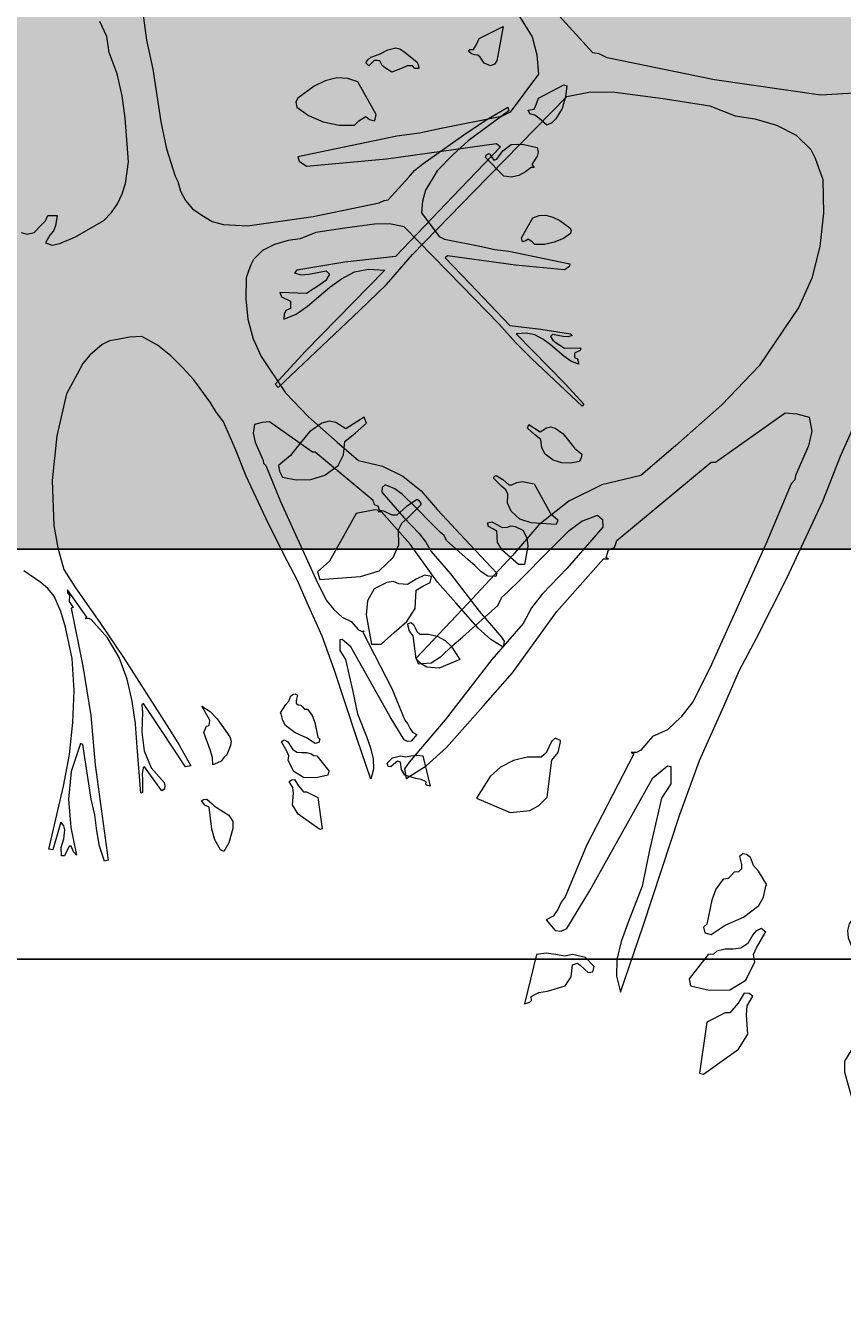
# Model space of a CAD drawing. Units: inches. Extents: x 84 to 1044, y -280 to 906.
# Tile 24 of 105: x 721 to 739, y -129 to -101. Entities that reach past the tile are written whole.
import ezdxf

# ---------------------------------------------------------------- set-up
doc = ezdxf.new("R2010")
doc.units = ezdxf.units.IN
for name, color, linetype, lineweight in [('A-ANNO-DIMS', 2, 'Continuous', 18), ('C-PROP', 7, 'Continuous', 25), ('L-PLNT', 114, 'Continuous', 15)]:
    doc.layers.add(name, color=color, linetype=linetype, lineweight=lineweight)
doc.layers.add('L-PLNT-PATT', color=9, linetype='Continuous', lineweight=9, true_color=0xafd9aa)
doc.styles.get("Standard").update_dxf_attribs({"font": 'arial.ttf'})
doc.dimstyles.get("Standard").update_dxf_attribs({"dimtxt": 0.18, "dimasz": 0.18, "dimexe": 0.18, "dimexo": 0.0625, "dimgap": 0.09, "dimtad": 0, "dimtih": 1, "dimtoh": 1, "dimdec": 4, "dimzin": 0, "dimdsep": 46, "dimtxsty": 'Standard', "dimcen": 0.09, "dimadec": 0, "dimazin": 0, "dimtfac": 1, "dimtdec": 4, "dimtofl": 0, "dimtmove": 0, "dimatfit": 3, "dimfxl": 1, "dimtolj": 1, "dimtzin": 0, "dimarcsym": 0})

# ---------------------------------------------------------------- blocks, each defined once
blk = doc.blocks.new('A$C37E508DF')
for p, q in [((0.7761, 1.2285), (0.7821, 1.1856)), ((0.7246, 1.1908), (0.7148, 1.2126)), ((1.2628, 1.1882), (1.2975, 1.2053)), ((1.2975, 1.2053), (1.2885, 1.1556)), ((0.7281, 1.168), (0.7246, 1.1908)), ((0.7821, 1.1856), (0.7911, 1.1436)), ((1.2589, 1.1792), (1.2628, 1.1882)), ((0.7396, 1.1371), (0.7281, 1.168)), ((1.1187, 1.1655), (1.1307, 1.1714)), ((1.1307, 1.1714), (1.1423, 1.1744)), ((1.1423, 1.1744), (1.1483, 1.1732)), ((1.1483, 1.1732), (1.1539, 1.1693)), ((1.1539, 1.1693), (1.1727, 1.1543)), ((1.2469, 1.1702), (1.2495, 1.1723)), ((1.2478, 1.1693), (1.2469, 1.1702)), ((1.2516, 1.1659), (1.2478, 1.1693)), ((1.2495, 1.1723), (1.2546, 1.1719)), ((1.2546, 1.1719), (1.2589, 1.1792)), ((1.099, 1.153), (1.102, 1.1573)), ((1.102, 1.1573), (1.1063, 1.1612)), ((1.1063, 1.1612), (1.1187, 1.1655)), ((1.2563, 1.1646), (1.2516, 1.1659)), ((1.2611, 1.1637), (1.2563, 1.1646)), ((1.2641, 1.1612), (1.2611, 1.1637)), ((1.2701, 1.1522), (1.2641, 1.1612)), ((1.1033, 1.1487), (1.099, 1.153)), ((1.111, 1.156), (1.1033, 1.1487)), ((1.1153, 1.1564), (1.111, 1.156)), ((1.1191, 1.1556), (1.1153, 1.1564)), ((1.1226, 1.1492), (1.1191, 1.1556)), ((1.1273, 1.1453), (1.1226, 1.1492)), ((1.1367, 1.1393), (1.1273, 1.1453)), ((1.1517, 1.1453), (1.1367, 1.1393)), ((1.1586, 1.1483), (1.1517, 1.1453)), ((1.1663, 1.1487), (1.1586, 1.1483)), ((1.1697, 1.1449), (1.1663, 1.1487)), ((1.1727, 1.1543), (1.1749, 1.1504)), ((1.1749, 1.1504), (1.1757, 1.1449)), ((1.2791, 1.1487), (1.2701, 1.1522)), ((1.2851, 1.1509), (1.2791, 1.1487)), ((1.2885, 1.1556), (1.2851, 1.1509)), ((0.7469, 1.1054), (0.7396, 1.1371)), ((0.7911, 1.1436), (0.8027, 1.0677)), ((1.1757, 1.1449), (1.1697, 1.1449)), ((1.3485, 1.102), (1.385, 1.1209)), ((1.385, 1.1209), (1.3897, 1.1196)), ((1.3897, 1.1196), (1.3875, 1.1037)), ((0.7512, 1.0728), (0.7469, 1.1054)), ((1.3455, 1.0934), (1.3485, 1.102)), ((1.3875, 1.1037), (1.3828, 1.087)), ((1.2713, 1.0694), (1.3044, 1.0887)), ((1.3044, 1.0887), (1.3057, 1.0835)), ((1.3421, 1.0861), (1.3455, 1.0934)), ((1.3057, 1.0835), (1.2469, 1.0402)), ((1.3335, 1.0844), (1.3421, 1.0861)), ((1.3361, 1.0793), (1.3335, 1.0844)), ((1.3434, 1.0771), (1.3361, 1.0793)), ((1.3828, 1.087), (1.3738, 1.072)), ((0.7538, 1.0415), (0.7512, 1.0728)), ((0.8027, 1.0677), (0.8108, 1.0287)), ((1.2409, 1.0488), (1.2713, 1.0694)), ((1.349, 1.0728), (1.3434, 1.0771)), ((1.3605, 1.063), (1.349, 1.0728)), ((1.3678, 1.0664), (1.3605, 1.063)), ((1.3738, 1.072), (1.3678, 1.0664)), ((1.1813, 1.0072), (1.2409, 1.0488)), ((0.7559, 1.0098), (0.7538, 1.0415)), ((1.2469, 1.0402), (1.2246, 1.0201)), ((1.2971, 1.0257), (1.3091, 1.0351)), ((1.3091, 1.0351), (1.3185, 1.0355)), ((1.3185, 1.0355), (1.3275, 1.0347)), ((1.3275, 1.0347), (1.3468, 1.0308)), ((0.8108, 1.0287), (0.8233, 0.9892)), ((1.2731, 1.0197), (1.2761, 1.0218)), ((1.2761, 1.0218), (1.2786, 1.0209)), ((1.2786, 1.0209), (1.2799, 1.0184)), ((1.2885, 1.0136), (1.2971, 1.0257)), ((1.3468, 1.0308), (1.3481, 1.0239)), ((1.3481, 1.0239), (1.3468, 1.018)), ((0.7516, 0.9785), (0.7559, 1.0098)), ((1.2246, 1.0201), (1.2023, 0.9969)), ((1.2718, 1.0162), (1.2731, 1.0197)), ((1.2984, 0.9892), (1.2718, 1.0162)), ((1.2799, 1.0184), (1.2842, 1.0124)), ((1.2842, 1.0124), (1.2885, 1.0136)), ((1.3468, 1.018), (1.3391, 1.0059)), ((1.1693, 0.9974), (1.1813, 1.0072)), ((1.3378, 1.0016), (1.3297, 0.9952)), ((1.3421, 1.0016), (1.3378, 1.0016)), ((1.3391, 1.0059), (1.3421, 1.0016)), ((0.8233, 0.9892), (0.8275, 0.9815)), ((1.1311, 0.9549), (1.1612, 0.9879)), ((1.1612, 0.9879), (1.1693, 0.9974)), ((1.2023, 0.9969), (1.1852, 0.9691)), ((1.3095, 0.9875), (1.2984, 0.9892)), ((1.3202, 0.9901), (1.3095, 0.9875)), ((1.3297, 0.9952), (1.3202, 0.9901)), ((0.7469, 0.9635), (0.7516, 0.9785)), ((0.8275, 0.9815), (0.8314, 0.9673)), ((0.8314, 0.9673), (0.8383, 0.954)), ((1.1852, 0.9691), (1.1809, 0.9532)), ((0.7401, 0.9493), (0.7469, 0.9635)), ((0.8383, 0.954), (0.8486, 0.942)), ((1.1183, 0.9506), (1.1256, 0.954)), ((1.1256, 0.954), (1.1311, 0.9549)), ((1.1809, 0.9532), (1.1796, 0.936)), ((0.7315, 0.9365), (0.7401, 0.9493)), ((0.8486, 0.942), (0.8619, 0.933)), ((1.0227, 0.9309), (1.1183, 0.9506)), ((0.6359, 0.9245), (0.6397, 0.9322)), ((0.6397, 0.9322), (0.653, 0.9322)), ((0.653, 0.9322), (0.6505, 0.9172)), ((0.7203, 0.9253), (0.7315, 0.9365)), ((0.8619, 0.933), (0.8769, 0.9236)), ((0.9279, 0.9172), (1.0227, 0.9309)), ((1.1796, 0.936), (1.2049, 0.9022)), ((1.3404, 0.9292), (1.3494, 0.9322)), ((1.3494, 0.9322), (1.3592, 0.9326)), ((1.3592, 0.9326), (1.3695, 0.93)), ((1.3695, 0.93), (1.3794, 0.9253)), ((0.6196, 0.9077), (0.6303, 0.9189)), ((0.6303, 0.9189), (0.6359, 0.9245)), ((0.6796, 0.9013), (0.7203, 0.9253)), ((0.8769, 0.9236), (0.8936, 0.9193)), ((0.8936, 0.9193), (0.9279, 0.9172)), ((1.1114, 0.9198), (1.0685, 0.9142)), ((1.1333, 0.9202), (1.1114, 0.9198)), ((1.1543, 0.9159), (1.1333, 0.9202)), ((1.3241, 0.9), (1.3404, 0.9292)), ((1.3794, 0.9253), (1.394, 0.9146)), ((0.6011, 0.9077), (0.6097, 0.9056)), ((0.6097, 0.9056), (0.6196, 0.9077)), ((0.6479, 0.9103), (0.6423, 0.9039)), ((0.6505, 0.9172), (0.6479, 0.9103)), ((1.0269, 0.9077), (1.0042, 0.8987)), ((1.0685, 0.9142), (1.0269, 0.9077)), ((1.2371, 0.8314), (1.1543, 0.9159)), ((1.394, 0.9146), (1.3957, 0.9112)), ((1.3957, 0.9112), (1.3948, 0.9065)), ((0.6384, 0.8974), (0.6359, 0.8927)), ((0.6423, 0.9039), (0.6384, 0.8974)), ((0.6569, 0.8919), (0.6796, 0.9013)), ((0.9866, 0.8962), (0.9673, 0.8906)), ((1.0042, 0.8987), (0.9866, 0.8962)), ((1.2049, 0.9022), (1.2126, 0.8983)), ((1.2126, 0.8983), (1.2662, 0.8876)), ((1.3254, 0.8944), (1.3241, 0.9)), ((1.3301, 0.8957), (1.3254, 0.8944)), ((1.3335, 0.8983), (1.3301, 0.8957)), ((1.3395, 0.8944), (1.3335, 0.8983)), ((1.3846, 0.8992), (1.3713, 0.8936)), ((1.3948, 0.9065), (1.3846, 0.8992)), ((0.6359, 0.8927), (0.6457, 0.8897)), ((0.6457, 0.8897), (0.6569, 0.8919)), ((0.9673, 0.8906), (0.9498, 0.8816)), ((1.2662, 0.8876), (1.2855, 0.8833)), ((1.3434, 0.8906), (1.3395, 0.8944)), ((1.3571, 0.8906), (1.3434, 0.8906)), ((1.3713, 0.8936), (1.3571, 0.8906)), ((0.9498, 0.8816), (0.9369, 0.8687)), ((1.2169, 0.8743), (1.2135, 0.8713)), ((1.3151, 0.8606), (1.2169, 0.8743)), ((1.2855, 0.8833), (1.3057, 0.8807)), ((1.3057, 0.8807), (1.394, 0.8623)), ((0.9369, 0.8687), (0.933, 0.861)), ((1.2135, 0.8713), (1.2491, 0.834)), ((1.394, 0.8623), (1.3927, 0.8584)), ((0.9296, 0.852), (0.9262, 0.8421)), ((0.933, 0.861), (0.9296, 0.852)), ((1.3863, 0.8541), (1.3151, 0.8606)), ((1.3927, 0.8584), (1.3863, 0.8541)), ((0.9262, 0.8421), (0.9257, 0.8121)), ((1.2919, 0.7752), (1.2371, 0.8314)), ((1.2491, 0.834), (1.3069, 0.7735)), ((0.9257, 0.8121), (0.9287, 0.7825)), ((0.9287, 0.7825), (0.936, 0.7542)), ((1.3151, 0.7487), (1.2919, 0.7752)), ((1.3069, 0.7735), (1.352, 0.7684)), ((1.3309, 0.7624), (1.3164, 0.7615)), ((1.3164, 0.7615), (1.3871, 0.6891)), ((1.3434, 0.7598), (1.3309, 0.7624)), ((1.355, 0.7538), (1.3434, 0.7598)), ((1.352, 0.7684), (1.3948, 0.7615)), ((1.3687, 0.7607), (1.3657, 0.7577)), ((1.3841, 0.7577), (1.3687, 0.7607)), ((1.3948, 0.7615), (1.397, 0.759)), ((0.7285, 0.7512), (0.7182, 0.7461)), ((0.7401, 0.7534), (0.7285, 0.7512)), ((0.7577, 0.7568), (0.7401, 0.7534)), ((0.7752, 0.7577), (0.7577, 0.7568)), ((0.798, 0.7452), (0.7752, 0.7577)), ((0.936, 0.7542), (0.9476, 0.7285)), ((1.3391, 0.7255), (1.3151, 0.7487)), ((1.3653, 0.7461), (1.355, 0.7538)), ((1.3657, 0.7577), (1.3691, 0.7521)), ((1.3691, 0.7521), (1.3743, 0.7482)), ((1.3914, 0.7572), (1.3841, 0.7577)), ((1.397, 0.759), (1.3914, 0.7572)), ((0.7182, 0.7461), (0.7002, 0.7307)), ((0.8173, 0.7298), (0.798, 0.7452)), ((1.3854, 0.7294), (1.3653, 0.7461)), ((1.3743, 0.7482), (1.3863, 0.7405)), ((1.3863, 0.7405), (1.4099, 0.7414)), ((1.4086, 0.7375), (1.4004, 0.7337)), ((1.4099, 0.7414), (1.4086, 0.7375)), ((0.7002, 0.7307), (0.6903, 0.7186)), ((0.8344, 0.7122), (0.8173, 0.7298)), ((0.9476, 0.7285), (0.9828, 0.6762)), ((1.3953, 0.7221), (1.3854, 0.7294)), ((1.4004, 0.7337), (1.4004, 0.7272)), ((1.4004, 0.7272), (1.4047, 0.7255)), ((0.6903, 0.7186), (0.6818, 0.7032)), ((1.4116, 0.6569), (1.3391, 0.7255)), ((1.4064, 0.7178), (1.3953, 0.7221)), ((1.4047, 0.7255), (1.406, 0.7221)), ((1.406, 0.7221), (1.4064, 0.7178)), ((0.6818, 0.7032), (0.6667, 0.6749)), ((0.8503, 0.6951), (0.8344, 0.7122)), ((0.8739, 0.6629), (0.8503, 0.6951)), ((1.3871, 0.6891), (1.4141, 0.6599)), ((0.6667, 0.6749), (0.6526, 0.614)), ((0.9828, 0.6762), (1.0162, 0.6415)), ((0.8824, 0.6492), (0.8739, 0.6629)), ((1.4141, 0.6599), (1.4116, 0.6569)), ((0.8932, 0.6342), (0.8824, 0.6492)), ((1.0162, 0.6415), (1.0574, 0.605)), ((0.9103, 0.5956), (0.8932, 0.6342)), ((0.9382, 0.6303), (0.936, 0.6179)), ((0.9493, 0.6333), (0.9382, 0.6303)), ((0.9596, 0.6342), (0.9493, 0.6333)), ((1.0218, 0.5904), (0.9596, 0.6342)), ((1.3327, 0.6252), (1.3348, 0.6303)), ((1.343, 0.6162), (1.3327, 0.6252)), ((1.3348, 0.6303), (1.3511, 0.62)), ((1.3511, 0.62), (1.3601, 0.6256)), ((1.3601, 0.6256), (1.3661, 0.6269)), ((1.3661, 0.6269), (1.3725, 0.6252)), ((1.3725, 0.6252), (1.3837, 0.6175)), ((0.6526, 0.614), (0.6457, 0.5497)), ((0.936, 0.6179), (0.939, 0.605)), ((1.352, 0.6089), (1.343, 0.6162)), ((1.3837, 0.6175), (1.3918, 0.6072)), ((0.939, 0.605), (0.9506, 0.5784)), ((1.0574, 0.605), (1.0883, 0.5784)), ((1.3533, 0.5969), (1.352, 0.6089)), ((1.3918, 0.6072), (1.4004, 0.5964)), ((0.9262, 0.5557), (0.9103, 0.5956)), ((1.0256, 0.5904), (1.0218, 0.5904)), ((1.1097, 0.5205), (1.0256, 0.5904)), ((1.358, 0.5874), (1.3533, 0.5969)), ((1.4004, 0.5964), (1.4111, 0.5874)), ((0.9506, 0.5784), (0.951, 0.5746)), ((1.0883, 0.5784), (1.123, 0.5703)), ((1.37, 0.5789), (1.358, 0.5874)), ((1.3824, 0.575), (1.37, 0.5789)), ((1.4103, 0.5823), (1.4077, 0.5771)), ((1.4111, 0.5874), (1.4103, 0.5823)), ((0.951, 0.5746), (0.9545, 0.5711)), ((0.9545, 0.5711), (0.9759, 0.5193)), ((1.123, 0.5703), (1.1526, 0.5557)), ((1.3953, 0.5746), (1.3824, 0.575)), ((1.4077, 0.5771), (1.3953, 0.5746)), ((0.9583, 0.4871), (0.9262, 0.5557)), ((1.1526, 0.5557), (1.1792, 0.5347)), ((1.2842, 0.554), (1.2855, 0.5557)), ((1.2855, 0.5557), (1.2876, 0.557)), ((1.2876, 0.557), (1.2971, 0.551)), ((0.6457, 0.5497), (0.6483, 0.4845)), ((1.2842, 0.5527), (1.2842, 0.554)), ((1.2958, 0.5407), (1.2842, 0.5527)), ((1.2971, 0.551), (1.3057, 0.5433)), ((1.3099, 0.5433), (1.3172, 0.5467)), ((1.3172, 0.5467), (1.3254, 0.548)), ((1.3254, 0.548), (1.3421, 0.5446)), ((1.3421, 0.5446), (1.3657, 0.5021)), ((1.1226, 0.5394), (1.1221, 0.5325)), ((1.1268, 0.5433), (1.1226, 0.5394)), ((1.141, 0.5377), (1.1268, 0.5433)), ((1.1521, 0.5296), (1.141, 0.5377)), ((1.1792, 0.5347), (1.2027, 0.5072)), ((1.3014, 0.536), (1.2958, 0.5407)), ((1.3044, 0.53), (1.3014, 0.536)), ((1.3057, 0.5433), (1.3099, 0.5433)), ((1.1221, 0.5325), (1.1539, 0.4961)), ((1.1706, 0.5111), (1.1521, 0.5296)), ((1.3039, 0.5167), (1.3044, 0.53)), ((0.9759, 0.5193), (1.0269, 0.4069)), ((1.1118, 0.5145), (1.1097, 0.5205)), ((1.117, 0.5124), (1.1118, 0.5145)), ((1.1191, 0.5055), (1.117, 0.5124)), ((1.1955, 0.4858), (1.1706, 0.5111)), ((1.3091, 0.5055), (1.3039, 0.5167)), ((1.117, 0.5042), (1.1191, 0.5055)), ((1.1217, 0.5042), (1.117, 0.5042)), ((1.1633, 0.4575), (1.1217, 0.5042)), ((1.2027, 0.5072), (1.2426, 0.4644)), ((1.3215, 0.4935), (1.3091, 0.5055)), ((1.3657, 0.5021), (1.3764, 0.4927)), ((1.1539, 0.4961), (1.1762, 0.4729)), ((1.2748, 0.4884), (1.2812, 0.4897)), ((1.2761, 0.4832), (1.2748, 0.4884)), ((1.2812, 0.4897), (1.2885, 0.4862)), ((1.3382, 0.4884), (1.3215, 0.4935)), ((1.3743, 0.4858), (1.3382, 0.4884)), ((1.3764, 0.4927), (1.3743, 0.4858)), ((0.6483, 0.4845), (0.6539, 0.4524)), ((0.9853, 0.4335), (0.9583, 0.4871)), ((1.207, 0.4747), (1.1955, 0.4858)), ((1.2825, 0.4798), (1.2761, 0.4832)), ((1.2885, 0.4764), (1.2825, 0.4798)), ((1.2885, 0.4862), (1.2962, 0.4815)), ((1.2894, 0.4601), (1.2885, 0.4764)), ((1.2962, 0.4815), (1.3039, 0.482)), ((1.3039, 0.482), (1.3087, 0.4841)), ((1.3087, 0.4841), (1.3147, 0.4832)), ((1.3147, 0.4832), (1.3258, 0.4777)), ((1.3258, 0.4777), (1.3318, 0.4669)), ((1.1762, 0.4729), (1.1856, 0.4605)), ((1.2122, 0.47), (1.207, 0.4747)), ((1.2156, 0.4627), (1.2122, 0.47)), ((1.3318, 0.4669), (1.3331, 0.4545)), ((1.2027, 0.4026), (1.1633, 0.4575)), ((1.1856, 0.4605), (1.1933, 0.4468)), ((1.2469, 0.4348), (1.2156, 0.4627)), ((1.2426, 0.4644), (1.2885, 0.4159)), ((1.2967, 0.4485), (1.2894, 0.4601)), ((1.3331, 0.4545), (1.3284, 0.4284)), ((0.6539, 0.4524), (0.6625, 0.4211)), ((1.1933, 0.4468), (1.2212, 0.4146)), ((1.3082, 0.4386), (1.2967, 0.4485)), ((1.0003, 0.4052), (0.9853, 0.4335)), ((1.2568, 0.4266), (1.2469, 0.4348)), ((1.3198, 0.4284), (1.3082, 0.4386)), ((0.6625, 0.4211), (0.6796, 0.3945)), ((1.2658, 0.4176), (1.2568, 0.4266)), ((1.3284, 0.4284), (1.3198, 0.4284)), ((0.6295, 0.4022), (0.6046, 0.4189)), ((1.2212, 0.4146), (1.2628, 0.361)), ((1.2752, 0.4116), (1.2658, 0.4176)), ((1.2868, 0.4108), (1.2752, 0.4116)), ((1.2885, 0.4159), (1.2868, 0.4108)), ((0.6397, 0.3936), (0.6295, 0.4022)), ((1.0145, 0.373), (1.0003, 0.4052)), ((1.0269, 0.4069), (1.0419, 0.3769)), ((1.2289, 0.373), (1.2027, 0.4026)), ((0.6487, 0.3825), (0.6397, 0.3936)), ((0.6959, 0.352), (0.668, 0.3919)), ((0.668, 0.3919), (0.668, 0.3872)), ((0.668, 0.3872), (0.6706, 0.3842)), ((0.6796, 0.3945), (0.7148, 0.3447)), ((0.6582, 0.3602), (0.6487, 0.3825)), ((0.6706, 0.3842), (0.6702, 0.3748)), ((0.6702, 0.3748), (0.6762, 0.3662)), ((1.0419, 0.3769), (1.0527, 0.3632)), ((0.6762, 0.3662), (0.6732, 0.3653)), ((0.6732, 0.3653), (0.6903, 0.2813)), ((1.0359, 0.3246), (1.0145, 0.373)), ((1.0527, 0.3632), (1.0647, 0.352)), ((1.2615, 0.3362), (1.2289, 0.373)), ((0.665, 0.3379), (0.6582, 0.3602)), ((0.6933, 0.3503), (0.6959, 0.352)), ((1.0647, 0.352), (1.078, 0.346)), ((1.2628, 0.361), (1.2949, 0.3233)), ((0.6985, 0.3503), (0.6933, 0.3503)), ((0.7023, 0.349), (0.6985, 0.3503)), ((0.7259, 0.3224), (0.7023, 0.349)), ((0.7148, 0.3447), (0.7487, 0.2937)), ((1.078, 0.346), (1.0883, 0.334)), ((1.1599, 0.3426), (1.1646, 0.3447)), ((1.1599, 0.3413), (1.1599, 0.3426)), ((1.162, 0.3319), (1.1599, 0.3413)), ((1.1646, 0.3447), (1.168, 0.3417)), ((1.168, 0.3417), (1.1702, 0.3366)), ((0.6745, 0.2924), (0.665, 0.3379)), ((1.0883, 0.334), (1.0921, 0.3319)), ((1.0921, 0.3319), (1.0968, 0.3319)), ((1.0968, 0.3319), (1.0947, 0.3306)), ((1.0947, 0.3306), (1.1367, 0.2491)), ((1.1676, 0.325), (1.162, 0.3319)), ((1.1702, 0.3366), (1.1727, 0.3314)), ((1.1727, 0.3314), (1.177, 0.3276)), ((1.2795, 0.3199), (1.2615, 0.3362)), ((0.7427, 0.2937), (0.7259, 0.3224)), ((1.0535, 0.2766), (1.0359, 0.3246)), ((1.0647, 0.3199), (1.0617, 0.3194)), ((1.0617, 0.3194), (1.0617, 0.304)), ((1.0711, 0.3147), (1.0647, 0.3199)), ((1.1719, 0.292), (1.1676, 0.325)), ((1.177, 0.3276), (1.1895, 0.3276)), ((1.1895, 0.3276), (1.2019, 0.3246)), ((1.2019, 0.3246), (1.2135, 0.3186)), ((1.2135, 0.3186), (1.2225, 0.3104)), ((1.2975, 0.3087), (1.2795, 0.3199)), ((1.2949, 0.3233), (1.2988, 0.3173)), ((1.0775, 0.3092), (1.0711, 0.3147)), ((1.1341, 0.2084), (1.0775, 0.3092)), ((1.2225, 0.3104), (1.2349, 0.2911)), ((1.2988, 0.3173), (1.2975, 0.3087)), ((1.0617, 0.304), (1.0698, 0.2911)), ((0.6775, 0.2465), (0.6745, 0.2924)), ((0.7542, 0.2628), (0.7427, 0.2937)), ((0.7487, 0.2937), (0.8151, 0.1899)), ((1.0698, 0.2911), (1.0805, 0.2448)), ((1.1792, 0.2847), (1.1719, 0.292)), ((1.1873, 0.28), (1.1792, 0.2847)), ((1.2349, 0.2911), (1.2049, 0.2783)), ((0.6903, 0.2813), (0.7015, 0.2101)), ((1.0861, 0.1775), (1.0535, 0.2766)), ((1.2049, 0.2783), (1.1873, 0.28)), ((0.7615, 0.2311), (0.7542, 0.2628)), ((0.6758, 0.2002), (0.6775, 0.2465)), ((0.9879, 0.2311), (0.9905, 0.2384)), ((0.9905, 0.2384), (0.9943, 0.241)), ((0.9943, 0.241), (0.9973, 0.2414)), ((0.9973, 0.2414), (1.0003, 0.2393)), ((1.0003, 0.2393), (0.9986, 0.232)), ((1.0805, 0.2448), (1.087, 0.2127)), ((1.1367, 0.2491), (1.1556, 0.2032)), ((0.7662, 0.1981), (0.7615, 0.2311)), ((0.7778, 0.2277), (0.7752, 0.2255)), ((0.8018, 0.1912), (0.7778, 0.2277)), ((0.9836, 0.226), (0.9879, 0.2311)), ((0.9986, 0.232), (0.9986, 0.2281)), ((0.9986, 0.2281), (1.0012, 0.2255)), ((0.7752, 0.2255), (0.7761, 0.2152)), ((0.8619, 0.2234), (0.8739, 0.2161)), ((0.87, 0.2101), (0.8619, 0.2234)), ((0.8739, 0.2161), (0.8841, 0.2054)), ((0.9759, 0.214), (0.9836, 0.226)), ((1.0012, 0.2255), (1.0051, 0.2251)), ((1.0051, 0.2251), (1.0076, 0.2225)), ((1.0076, 0.2225), (1.0106, 0.2195)), ((1.0106, 0.2195), (1.0149, 0.2191)), ((1.0149, 0.2191), (1.0214, 0.2101)), ((0.7015, 0.2101), (0.7079, 0.1389)), ((0.7761, 0.2152), (0.7752, 0.1861)), ((0.8734, 0.2032), (0.87, 0.2101)), ((0.8841, 0.2054), (0.9026, 0.1792)), ((0.9768, 0.2127), (0.9759, 0.214)), ((0.9789, 0.2028), (0.9768, 0.2127)), ((1.0214, 0.2101), (1.0252, 0.2002)), ((1.087, 0.2127), (1.0998, 0.1797)), ((1.1543, 0.1749), (1.1341, 0.2084)), ((0.6706, 0.1539), (0.6758, 0.2002)), ((0.7688, 0.1646), (0.7662, 0.1981)), ((0.8649, 0.1857), (0.8687, 0.1947)), ((0.8687, 0.1947), (0.8726, 0.1955)), ((0.8726, 0.1955), (0.8734, 0.2032)), ((0.9832, 0.1955), (0.9789, 0.2028)), ((0.9969, 0.1852), (0.9832, 0.1955)), ((1.0252, 0.2002), (1.0295, 0.1788)), ((1.1556, 0.2032), (1.1594, 0.1985)), ((1.1594, 0.1985), (1.1624, 0.1921)), ((0.7752, 0.1861), (0.7787, 0.1591)), ((0.8383, 0.1359), (0.8018, 0.1912)), ((0.8151, 0.1899), (0.8288, 0.1685)), ((0.8743, 0.1608), (0.8649, 0.1857)), ((1.0132, 0.1779), (0.9969, 0.1852)), ((1.1624, 0.1921), (1.1663, 0.1861)), ((1.1727, 0.1827), (1.1646, 0.1732)), ((1.1663, 0.1861), (1.1727, 0.1827)), ((0.9026, 0.1792), (0.9043, 0.1732)), ((0.9043, 0.1732), (0.9035, 0.1668)), ((0.9768, 0.1719), (0.9811, 0.1749)), ((0.9776, 0.1711), (0.9768, 0.1719)), ((0.9853, 0.1578), (0.9776, 0.1711)), ((0.9811, 0.1749), (0.9858, 0.1728)), ((0.9858, 0.1728), (0.9884, 0.1694)), ((1.0256, 0.1698), (1.0132, 0.1779)), ((1.0312, 0.1711), (1.0256, 0.1698)), ((1.0295, 0.1788), (1.0325, 0.1762)), ((1.0325, 0.1762), (1.0312, 0.1711)), ((1.1063, 0.1183), (1.0861, 0.1775)), ((1.0998, 0.1797), (1.1058, 0.1634)), ((1.1594, 0.1728), (1.1543, 0.1749)), ((1.1646, 0.1732), (1.1594, 0.1728)), ((0.6865, 0.1698), (0.6732, 0.1295)), ((0.6903, 0.1681), (0.6865, 0.1698)), ((0.7023, 0.0892), (0.6903, 0.1681)), ((0.774, 0.0982), (0.7688, 0.1646)), ((0.7787, 0.1591), (0.789, 0.1346)), ((0.8288, 0.1685), (0.846, 0.1376)), ((0.8777, 0.1496), (0.8743, 0.1608)), ((0.9035, 0.1668), (0.8983, 0.1535)), ((0.9884, 0.1694), (0.9931, 0.1616)), ((0.9931, 0.1616), (0.9991, 0.1574)), ((1.1058, 0.1634), (1.1097, 0.1475)), ((0.662, 0.108), (0.6706, 0.1539)), ((0.8781, 0.1389), (0.8777, 0.1496)), ((0.894, 0.1496), (0.8902, 0.1441)), ((0.8983, 0.1535), (0.894, 0.1496)), ((0.9879, 0.1518), (0.9853, 0.1578)), ((0.9866, 0.1453), (0.9879, 0.1518)), ((0.9991, 0.1574), (1.0059, 0.1565)), ((1.0059, 0.1565), (1.0132, 0.1565)), ((1.0132, 0.1565), (1.0205, 0.1548)), ((1.0205, 0.1548), (1.0235, 0.1522)), ((1.0235, 0.1522), (1.0282, 0.1518)), ((1.0282, 0.1518), (1.0454, 0.1303)), ((1.1097, 0.1475), (1.1101, 0.1325)), ((1.1298, 0.1411), (1.1376, 0.1492)), ((1.1376, 0.1492), (1.1491, 0.1518)), ((1.1491, 0.1518), (1.1564, 0.1505)), ((1.1564, 0.1505), (1.1642, 0.1518)), ((1.1642, 0.1518), (1.1727, 0.1531)), ((1.1727, 0.1531), (1.1813, 0.1518)), ((1.1813, 0.1518), (1.192, 0.108)), ((0.7079, 0.1389), (0.7268, 0.0013)), ((0.846, 0.1376), (0.8383, 0.1359)), ((0.8846, 0.1419), (0.8781, 0.1389)), ((0.8902, 0.1441), (0.8846, 0.1419)), ((0.9948, 0.1291), (0.9866, 0.1453)), ((1.1311, 0.1364), (1.1298, 0.1411)), ((1.1354, 0.1359), (1.1311, 0.1364)), ((1.1384, 0.1389), (1.1354, 0.1359)), ((1.1423, 0.1423), (1.1384, 0.1389)), ((1.1449, 0.1441), (1.1423, 0.1423)), ((1.1491, 0.1428), (1.1449, 0.1441)), ((1.1504, 0.132), (1.1491, 0.1428)), ((0.6732, 0.1295), (0.6693, 0.0892)), ((0.7774, 0.1346), (0.7757, 0.1261)), ((0.7757, 0.1261), (0.7761, 0.117)), ((0.7791, 0.1359), (0.7774, 0.1346)), ((0.8044, 0.1012), (0.7791, 0.1359)), ((0.789, 0.1346), (0.8074, 0.1132)), ((1.0089, 0.1205), (0.9948, 0.1291)), ((1.0454, 0.1303), (1.0441, 0.1239)), ((1.1101, 0.1325), (1.1063, 0.1183)), ((1.1556, 0.1239), (1.1504, 0.132)), ((0.7761, 0.117), (0.7761, 0.099)), ((0.9884, 0.1149), (0.9918, 0.117)), ((0.9935, 0.1063), (0.9884, 0.1149)), ((0.9918, 0.117), (0.9961, 0.1175)), ((0.9961, 0.1175), (1.0016, 0.1085)), ((1.0274, 0.12), (1.0089, 0.1205)), ((1.0441, 0.1239), (1.0274, 0.12)), ((1.1714, 0.1192), (1.1556, 0.1239)), ((1.1792, 0.1179), (1.1714, 0.1192)), ((1.186, 0.1145), (1.1792, 0.1179)), ((1.1856, 0.111), (1.186, 0.1145)), ((0.641, 0.0172), (0.662, 0.108)), ((0.8083, 0.1037), (0.8044, 0.1012)), ((0.8074, 0.1132), (0.8087, 0.1089)), ((0.8087, 0.1089), (0.8083, 0.1037)), ((0.9943, 0.0982), (0.9935, 0.1063)), ((1.0016, 0.1085), (1.0089, 0.0999)), ((1.1873, 0.1093), (1.1856, 0.111)), ((1.192, 0.108), (1.1873, 0.1093)), ((0.7761, 0.099), (0.774, 0.0982)), ((0.9931, 0.081), (0.9943, 0.0982)), ((1.0089, 0.0999), (1.0132, 0.0999)), ((1.0132, 0.0999), (1.0295, 0.0917)), ((1.0295, 0.0917), (1.0359, 0.0463)), ((0.6693, 0.0892), (0.6728, 0.0484)), ((0.7075, 0.0665), (0.7023, 0.0892)), ((0.8619, 0.0875), (0.8649, 0.0887)), ((0.8619, 0.0866), (0.8619, 0.0875)), ((0.8666, 0.0806), (0.8619, 0.0866)), ((0.8649, 0.0887), (0.8691, 0.0892)), ((0.8726, 0.0776), (0.8666, 0.0806)), ((0.8691, 0.0892), (0.8769, 0.0827)), ((0.8769, 0.0827), (0.8799, 0.0797)), ((0.8799, 0.0797), (0.8893, 0.0733)), ((1.0012, 0.0677), (0.9931, 0.081)), ((0.8764, 0.0459), (0.8726, 0.0776)), ((0.8893, 0.0733), (0.9013, 0.066)), ((0.7105, 0.0437), (0.7075, 0.0665)), ((0.9013, 0.066), (0.9069, 0.057)), ((0.9069, 0.057), (0.9069, 0.0471)), ((1.0325, 0.0454), (1.0012, 0.0677)), ((0.6582, 0.0562), (0.6466, 0.0159)), ((0.6625, 0.051), (0.6582, 0.0562)), ((0.6642, 0.045), (0.6625, 0.051)), ((0.6728, 0.0484), (0.6809, 0.0082)), ((0.8807, 0.0304), (0.8764, 0.0459)), ((0.9069, 0.0471), (0.9009, 0.0261)), ((1.0359, 0.0463), (1.0325, 0.0454)), ((0.6625, 0.0321), (0.6642, 0.045)), ((0.7144, 0.0214), (0.7105, 0.0437)), ((0.659, 0.0193), (0.6625, 0.0321)), ((0.8889, 0.0159), (0.8807, 0.0304)), ((0.9009, 0.0261), (0.894, 0.0137)), ((0.6466, 0.0159), (0.641, 0.0172)), ((0.6595, 0.0077), (0.659, 0.0193)), ((0.6702, 0.0214), (0.6637, 0.0077)), ((0.6732, 0.0214), (0.6702, 0.0214)), ((0.6766, 0.0133), (0.6732, 0.0214)), ((0.6809, 0.0082), (0.6766, 0.0133)), ((0.7216, 0), (0.7144, 0.0214)), ((0.894, 0.0137), (0.8889, 0.0159)), ((0.6637, 0.0077), (0.6595, 0.0077)), ((0.7268, 0.0013), (0.7216, 0))]:
    blk.add_line(p, q)
blk = doc.blocks.new('*D60')
at = {"layer": 'A-ANNO-DIMS', "color": 0, "lineweight": -2, "transparency": 16777216}
for p, q in [((134.179, -121.942), (134.179, -180.64)), ((992.074, -121.942), (992.074, -180.64)), ((134.359, -180.46), (562.733, -180.46)), ((991.894, -180.46), (563.521, -180.46))]:
    blk.add_line(p, q, dxfattribs=at)
at = {"layer": 'A-ANNO-DIMS', "color": 0, "transparency": 16777216}
for points in [[(134.359, -180.43), (134.359, -180.49), (134.179, -180.46)], [(991.894, -180.43), (991.894, -180.49), (992.074, -180.46)]]:
    blk.add_solid(points, dxfattribs=at)
at = {"layer": 'Defpoints', "color": 0, "transparency": 16777216}
for p in [(134.179, -121.88), (992.074, -121.88), (992.074, -180.46)]:
    blk.add_point(p, dxfattribs=at)
at = {"layer": 'A-ANNO-DIMS', "color": 0, "transparency": 16777216, "insert": (563.127, -180.46), "char_height": 0.18, "attachment_point": 5}
blk.add_mtext('\\A1;857.9', dxfattribs=at)

msp = doc.modelspace()

# ---------------------------------------------------------------- hatches: boundary and pattern name
at = {"layer": 'L-PLNT-PATT', "transparency": 33554597}
h = msp.add_hatch(color=256, dxfattribs=at)
h.dxf.hatch_style = 1
h.paths.add_polyline_path([(791.074, 31.12), (791.074, 91.12), (743.074, 91.12), (674.074, 91.12), (674.074, 31.12), (650.074, 31.12), (650.074, -112.88), (983.074, -112.88), (983.074, -64.88), (791.074, -64.88)])

# ---------------------------------------------------------------- linework, layer by layer
at = {"layer": 'C-PROP'}
for points in [[(143.179, -121.88), (134.179, -121.88), (134.179, 856.12), (992.074, 856.12), (992.074, -121.88), (624.574, -121.88)], [(143.179, -112.88), (143.179, 847.12), (983.074, 847.12), (983.074, -112.88), (624.574, -112.88)]]:
    msp.add_lwpolyline(points, dxfattribs=at)

# ---------------------------------------------------------------- block references
at = {"layer": 'L-PLNT'}
for p, xscale, yscale, zscale in [((761.712, -125.52), -24.64361536662419, 24.64361536662419, 24.64361536662419), ((712.152, -119.725, 0), 15.19586232982809, 15.19586232982809, 15.19586232982809)]:
    msp.add_blockref('A$C37E508DF', p, dxfattribs=dict(at, xscale=xscale, yscale=yscale, zscale=zscale))

# ---------------------------------------------------------------- dimensions: what is measured, and where the dimension line sits
at = {"layer": 'A-ANNO-DIMS'}
dim = msp.add_linear_dim(base=(992.074, -180.46), p1=(134.179, -121.88), p2=(992.074, -121.88), dimstyle='Standard', override={"dimdec": 1, "dimlfac": 1, "dimrnd": 0, "dimzin": 0, "dimdsep": 46, "dimlunit": 2}, dxfattribs=at)
dim.commit()
dim.dimension.update_dxf_attribs({"geometry": '*D60', "text_midpoint": (563.127, -180.46)})

doc.saveas('drawing.dxf')
